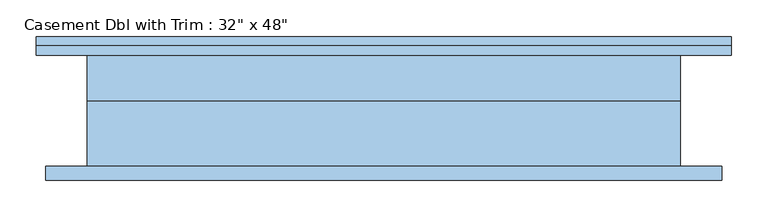
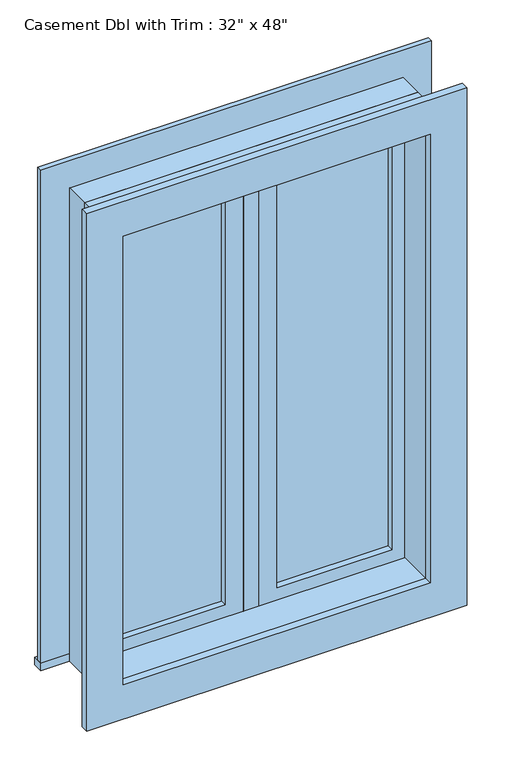
"""IFC4 building model written with IfcOpenShell, lengths in millimetres: window geometry."""

from ifc_helpers import new_model, si_unit, frame, origin, place, context, project, spatial, polyline, outline, extrude, source, transform, mapped, element, save


def window_02f8983a(model_context):
    return source(origin(), model_context, "Body", "SweptSolid", [
        extrude(outline(polyline([(63.5, 60.325), (342.9, 60.325), (342.9, 47.625), (63.5, 47.625), (63.5, 60.325)])), frame((0.0, 0.0, 977.9), z_axis=(0.0, 0.0, 1.0), x_axis=(1.0, 0.0, 0.0)), (0.0, 0.0, 1.0), 1092.2),
        extrude(outline(polyline([(2114.55, 19.05), (933.45, 19.05), (933.45, 387.35), (2114.55, 387.35), (2114.55, 19.05)]), holes=[polyline([(2070.1, 63.5), (2070.1, 342.9), (977.9, 342.9), (977.9, 63.5), (2070.1, 63.5)])]), frame((0.0, 31.75, 0.0), z_axis=(0.0, 1.0, 0.0), x_axis=(0.0, 0.0, 1.0)), (0.0, 0.0, 1.0), 44.45),
        extrude(outline(polyline([(19.05, 31.75), (-19.05, 31.75), (-19.05, 95.25), (19.05, 95.25), (19.05, 31.75)])), frame((0.0, 0.0, 933.45), z_axis=(0.0, 0.0, 1.0), x_axis=(1.0, 0.0, 0.0)), (0.0, 0.0, 1.0), 1181.1),
        extrude(outline(polyline([(-476.25, 120.65), (476.25, 120.65), (476.25, 95.25), (-476.25, 95.25), (-476.25, 120.65)])), frame((0.0, 0.0, 914.4), z_axis=(0.0, 0.0, 1.0), x_axis=(1.0, 0.0, 0.0)), (0.0, 0.0, 1.0), 19.05),
        extrude(outline(polyline([(2114.55, -387.35), (2114.55, 387.35), (933.45, 387.35), (933.45, 476.25), (2203.45, 476.25), (2203.45, -476.25), (933.45, -476.25), (933.45, -387.35), (2114.55, -387.35)])), frame((0.0, 95.25, 0.0), z_axis=(0.0, 1.0, 0.0), x_axis=(0.0, 0.0, 1.0)), (0.0, 0.0, 1.0), 12.7),
        extrude(outline(polyline([(2190.75, 463.55), (2190.75, -463.55), (857.25, -463.55), (857.25, 463.55), (2190.75, 463.55)]), holes=[polyline([(2101.85, 374.65), (946.15, 374.65), (946.15, -374.65), (2101.85, -374.65), (2101.85, 374.65)])]), frame((0.0, -76.2, 0.0), z_axis=(0.0, 1.0, 0.0), x_axis=(0.0, 0.0, 1.0)), (0.0, 0.0, 1.0), 19.05),
        extrude(outline(polyline([(-63.5, 47.625), (-342.9, 47.625), (-342.9, 60.325), (-63.5, 60.325), (-63.5, 47.625)])), frame((0.0, 0.0, 977.9), z_axis=(0.0, 0.0, 1.0), x_axis=(1.0, 0.0, 0.0)), (0.0, 0.0, 1.0), 1092.2),
        extrude(outline(polyline([(2114.55, -387.35), (933.45, -387.35), (933.45, -19.05), (2114.55, -19.05), (2114.55, -387.35)]), holes=[polyline([(2070.1, -342.9), (2070.1, -63.5), (977.9, -63.5), (977.9, -342.9), (2070.1, -342.9)])]), frame((0.0, 31.75, 0.0), z_axis=(0.0, 1.0, 0.0), x_axis=(0.0, 0.0, 1.0)), (0.0, 0.0, 1.0), 44.45),
        extrude(outline(polyline([(2133.6, -406.4), (914.4, -406.4), (914.4, 406.4), (2133.6, 406.4), (2133.6, -406.4)]), holes=[polyline([(2101.85, -374.65), (2101.85, 374.65), (946.15, 374.65), (946.15, -374.65), (2101.85, -374.65)])]), frame((0.0, -57.15, 0.0), z_axis=(0.0, 1.0, 0.0), x_axis=(0.0, 0.0, 1.0)), (0.0, 0.0, 1.0), 88.9),
        extrude(outline(polyline([(2133.6, 406.4), (2133.6, -406.4), (914.4, -406.4), (914.4, 406.4), (2133.6, 406.4)]), holes=[polyline([(2114.55, 387.35), (933.45, 387.35), (933.45, -387.35), (2114.55, -387.35), (2114.55, 387.35)])]), frame((0.0, 31.75, 0.0), z_axis=(0.0, 1.0, 0.0), x_axis=(0.0, 0.0, 1.0)), (0.0, 0.0, 1.0), 63.5),
    ])


if __name__ == "__main__":
    model = new_model("IFC4")
    model_context = context("Model", 3, world=origin())
    ifc_project = project(units=[si_unit("LENGTHUNIT", "METRE", prefix="MILLI")], contexts=[model_context])
    site = spatial("IfcSite", under=ifc_project)
    building = spatial("IfcBuilding", under=site)
    placement = place(None, origin())
    window_shape = window_02f8983a(model_context)
    element("IfcWindow", 1, ObjectType="Casement Dbl with Trim : 32\" x 48\"", at=placement, inside=building, context=model_context, shape_type="MappedRepresentation", body=[
        mapped(window_shape, transform((0.0, 0.0, 0.0), x_axis=(1.0, 0.0, 0.0), y_axis=(0.0, 1.0, 0.0), z_axis=(0.0, 0.0, 1.0))),
    ])
    save(model, "model.ifc")

# Revit data of these elements
# Type "Casement Dbl with Trim : 32\" x 48\""
#   Type Mark = "15"
#   Construction Type Id = "GSP4R"
#   Assembly Code = "B2020100"
#   Analytic Construction = "1/8 in Pilkington single glazing"
#   Visual Light Transmittance = 0.9
#   Solar Heat Gain Coefficient = 0.78
#   Heat Transfer Coefficient (U) = 0.6496 BTU/(h·ft²·°F)
#   Height = 4' - 0"
#   Default Sill Height = 3' - 0"
#   Trim Projection - Ext. = 0' - 0 1/2"
#   Trim Projection - Int. = 0' - 0 3/4"
#   Trim Width - Exterior = 0' - 3 1/2"
#   Trim Width - Interior = 0' - 3 1/2"
#   Width = 2' - 8"
#   Window Inset = 0' - 0 3/4"
#   Define Thermal Properties by = 1
#   Glass Pane Material = Glass
#   Sash Material = Sash
#   Trim Exterior Material = Trim
#   Trim Interior Material = Trim
#   Wall Closure = (empty or 0)
# Element 1 (IfcWindow, "Casement Dbl with Trim : 32\" x 48\"")
#   Materials on its faces: "Sash", "Trim", "Glass"
# Materials
#   "Glass": class "Glass", colour RGB 0 128 192, transparency 0.75, Description = "Soda Lime Glass", Cost = 0
#   "Sash": class "Wood", colour RGB 224 178 126, transparency 0
#   "Trim": class "Wood", colour RGB 224 178 126, transparency 0
